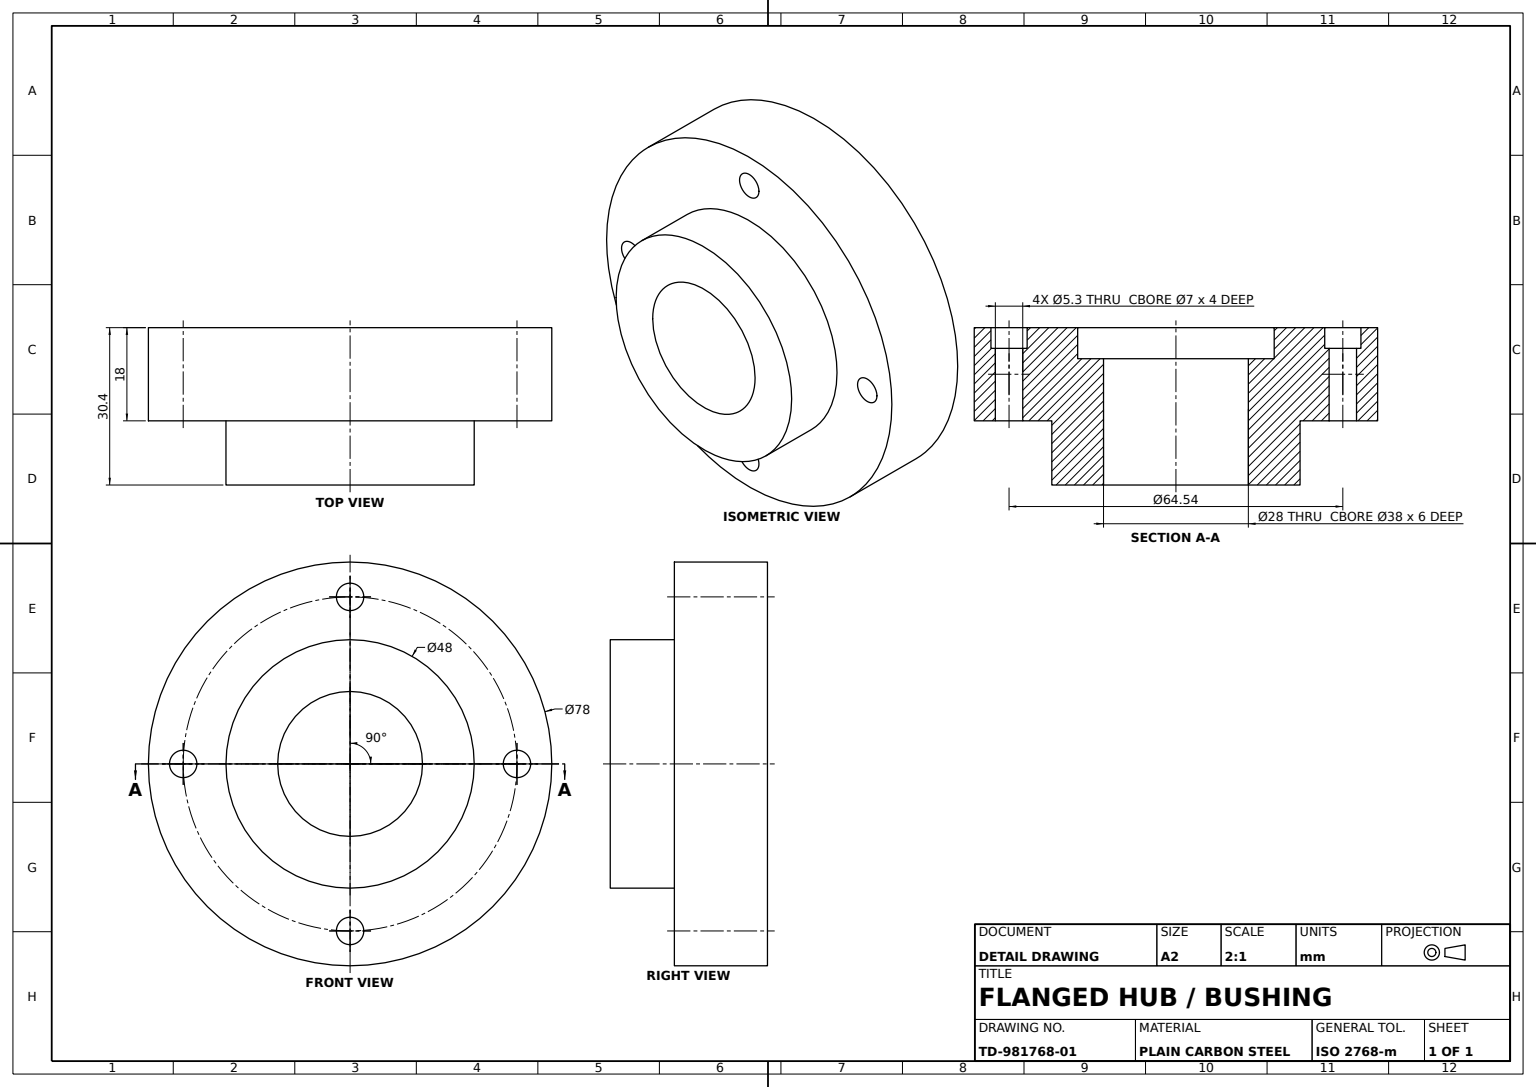
SolidWorks part; units mm, degrees
material "Plain Carbon Steel"
ref_plane "Front Plane" through (0, 0, 0) normal (0, 0, 1) x (1, 0, 0)
ref_plane "Top Plane" through (0, 0, 0) normal (0, 1, 0) x (1, 0, 0)
ref_plane "Right Plane" through (0, 0, 0) normal (1, 0, 0) x (0, 0, -1)
sketch "Hub Profile Sketch" plane through (0, 0, 0) normal (0, 0, 1) x (1, 0, 0)
  line L0 (9, -24) -> (9, -39)
  line L3 (-9, -39) -> (9, -39)
  line L5 (-9, 0) -> (21.4, 0)
  line L6 (-9, -39) -> (-4.3846, -19) construction
  line L9 (9, -24) -> (21.4, -24)
  line L10 (21.4, 0) -> (21.4, -24)
  line L11 (6.6, 0) -> (57.7329, 0) construction
  line L13 (-9, 0) -> (-9, -19)
  line L14 (-9, -19) -> (4.6, -19)
  line L15 (6.6, 0) -> (6.6, -17)
  line L24 (-9, 0) -> (-70.1947, 0) construction
  line L25 (-5, -19) -> (0, -19)
  line L26 (-5, -19) -> (-5, -39)
  line L27 (-5, -39) -> (0, -39)
  line L28 (0, -19) -> (0, -39)
  line L29 (-9, 0) -> (-9, -39)
  line L30 (4.3846, -19) -> (9, -39) construction
  arc A0 (6.6, -17) -> (4.6, -19) centre (4.6, -17) cw
  point P0 (0, 0)
  point P17 (6.6, -19)
  point P20 (6.6, 19)
  dimension "D7" = 2
  dimension "D2" = 18
  dimension "D3" = 15.6
  dimension "D4" = 24
  dimension "D5" = 38
  dimension "D6" = 19
  dimension "D8" = 30.4
  dimension "D9" = 15
  dimension "D13" = 5
revolve "Flanged Hub Body" add sketch "Hub Profile Sketch" angle 360 about L11
sketch "Mounting Holes Sketch" plane through (21.4, 0, 0) normal (1, 0, 0) x (0, 0, -1)
  circle A0 centre (0, 0) radius 14
  circle A1 centre (0, 32.2694) radius 2.65
  circle A2 centre (32.2694, 0) radius 2.65
  circle A3 centre (0, -32.2694) radius 2.65
  circle A4 centre (-32.2694, 0) radius 2.65
  circle A5 centre (0, 0) radius 24 construction
  point P13 (0, 0)
  dimension "D1" = 28
  dimension "D2" = 5.3
  dimension "D4" = 32.2694
  dimension "D3" = 4
extrude "Mounting Holes 4xØ5.3" cut sketch "Mounting Holes Sketch" against normal blind 317
sketch "Slot Sketch" plane through (-9, 0, 0) normal (-1, 0, 0) x (0, 0, 1)
  circle A0 centre (0, 32.2694) radius 3.5
  circle A1 centre (-32.2694, 0) radius 3.5
  circle A2 centre (0, -32.2694) radius 3.5
  circle A3 centre (32.2694, 0) radius 3.5
  dimension "D1" = 7
extrude "Slot 7mm x 4 Deep" cut sketch "Slot Sketch" against normal blind 4
sketch "Recess Sketch" plane through (-9, 0, 0) normal (-1, 0, 0) x (0, 0, 1)
  circle A0 centre (0, 0) radius 19
  dimension "D1" = 38
extrude "Recess Ø38 x 6 Deep" cut sketch "Recess Sketch" against normal blind 6
